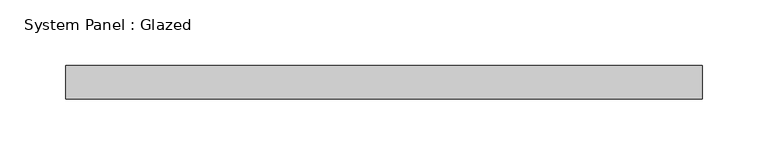
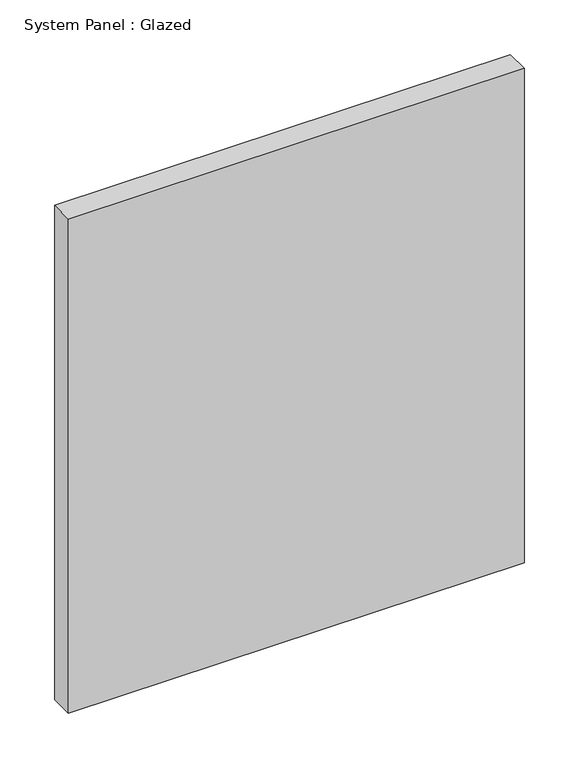
"""IFC4 building model written with IfcOpenShell, lengths in millimetres: plate geometry, System Panel : Glazed."""

from ifc_helpers import new_model, si_unit, origin, origin_with_axes, place, context, project, spatial, polyline, outline, extrude, source, transform, mapped, element, save


def system_panel_glazed_0ac8c76b(model_context):
    return source(origin(), model_context, "Body", "SweptSolid", [
        extrude(outline(polyline([(241.3, 19.05), (-241.3, 19.05), (-241.3, 44.45), (241.3, 44.45), (241.3, 19.05)])), origin_with_axes(), (0.0, 0.0, 1.0), 553.1636426),
    ])


if __name__ == "__main__":
    model = new_model("IFC4")
    model_context = context("Model", 3, world=origin())
    ifc_project = project(units=[si_unit("LENGTHUNIT", "METRE", prefix="MILLI")], contexts=[model_context])
    site = spatial("IfcSite", under=ifc_project)
    building = spatial("IfcBuilding", under=site)
    placement = place(None, origin())
    system_panel_glazed_shape = system_panel_glazed_0ac8c76b(model_context)
    element("IfcPlate", 1, ObjectType="System Panel : Glazed", at=placement, inside=building, context=model_context, shape_type="MappedRepresentation", body=[
        mapped(system_panel_glazed_shape, transform((0.0, 0.0, 0.0), x_axis=(1.0, 0.0, 0.0), y_axis=(0.0, 1.0, 0.0), z_axis=(0.0, 0.0, 1.0))),
    ])
    save(model, "model.ifc")

# Revit data of these elements
# Type "System Panel : Glazed"
#   Construction Type Id = "GSP4R"
#   Analytic Construction = "1/8 in Pilkington single glazing"
#   Visual Light Transmittance = 0.9
#   Solar Heat Gain Coefficient = 0.86
#   Heat Transfer Coefficient (U) = 1.18115 BTU/(h·ft²·°F)
#   Define Thermal Properties by = 1
# Element 1 (IfcPlate, "System Panel : Glazed")
#   Materials on its faces: "Glass"
# Materials
#   "Glass": class "Glass", colour RGB 0 128 192, transparency 0.75, Description = "Soda Lime Glass", Cost = 0
